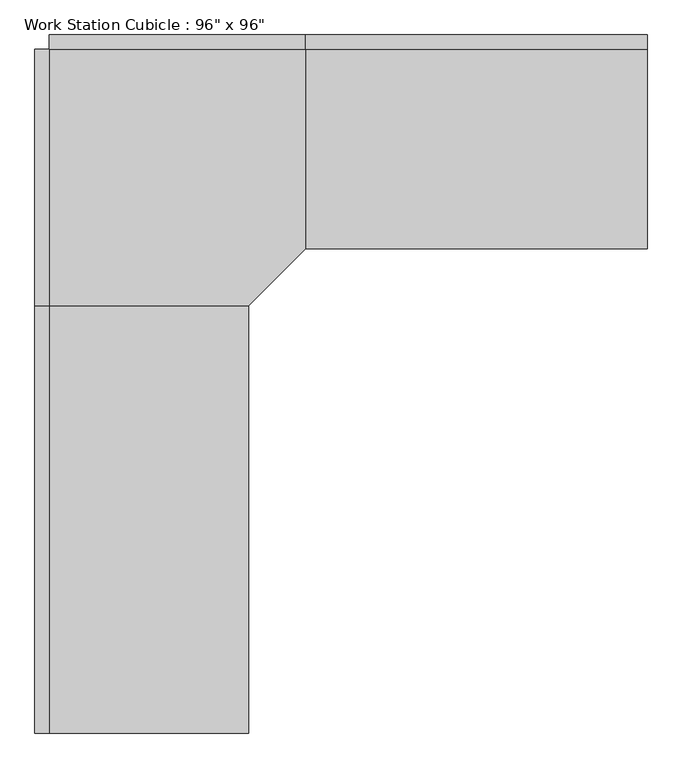
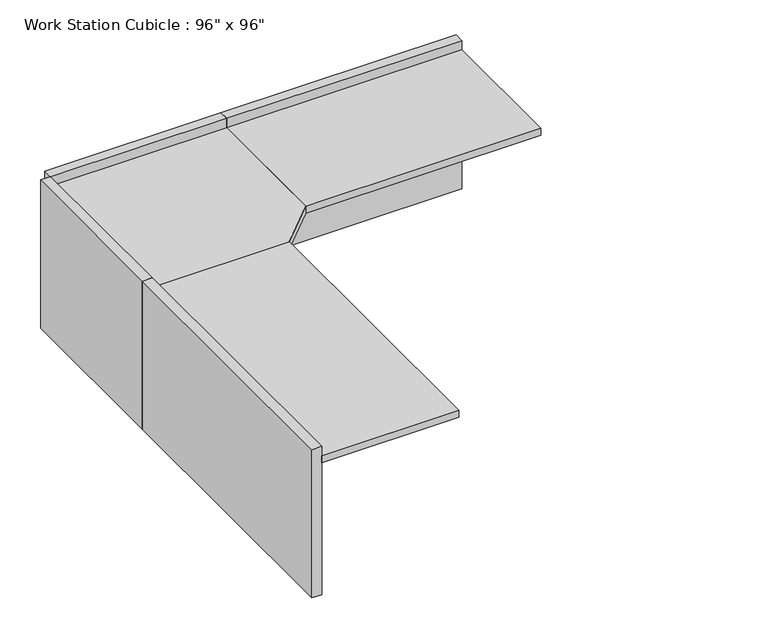
"""IFC4 building model written with IfcOpenShell, lengths in millimetres: furniture geometry."""

from ifc_helpers import new_model, si_unit, frame, origin, origin_with_axes, place, context, project, spatial, polyline, outline, extrude, source, transform, mapped, element, save


def furniture_3226db35(model_context):
    return source(origin(), model_context, "Body", "SweptSolid", [
        extrude(outline(polyline([(-80.9317522, -545.8230076), (833.4682478, -545.8230076), (833.4682478, -1257.0230076), (630.2682478, -1460.2230076), (-80.9317522, -1460.2230076), (-80.9317522, -545.8230076)])), frame((0.0, 0.0, 723.9), z_axis=(0.0, 0.0, 1.0), x_axis=(1.0, 0.0, 0.0)), (0.0, 0.0, 1.0), 38.1),
        extrude(outline(polyline([(630.2682478, -2984.2230076), (-80.9317522, -2984.2230076), (-80.9317522, -1460.2230076), (630.2682478, -1460.2230076), (630.2682478, -2984.2230076)])), frame((0.0, 0.0, 723.9), z_axis=(0.0, 0.0, 1.0), x_axis=(1.0, 0.0, 0.0)), (0.0, 0.0, 1.0), 38.1),
        extrude(outline(polyline([(2052.6682478, -1257.0230076), (833.4682478, -1257.0230076), (833.4682478, -545.8230076), (2052.6682478, -545.8230076), (2052.6682478, -1257.0230076)])), frame((0.0, 0.0, 723.9), z_axis=(0.0, 0.0, 1.0), x_axis=(1.0, 0.0, 0.0)), (0.0, 0.0, 1.0), 38.1),
        extrude(outline(polyline([(2052.6682478, -545.8230076), (833.4682478, -545.8230076), (833.4682478, -495.0230076), (2052.6682478, -495.0230076), (2052.6682478, -545.8230076)])), origin_with_axes(), (0.0, 0.0, 1.0), 812.8),
        extrude(outline(polyline([(833.4682478, -545.8230076), (-80.9317522, -545.8230076), (-80.9317522, -495.0230076), (833.4682478, -495.0230076), (833.4682478, -545.8230076)])), origin_with_axes(), (0.0, 0.0, 1.0), 812.8),
        extrude(outline(polyline([(-80.9317522, -1460.2230076), (-131.7317522, -1460.2230076), (-131.7317522, -545.8230076), (-80.9317522, -545.8230076), (-80.9317522, -1460.2230076)])), origin_with_axes(), (0.0, 0.0, 1.0), 812.8),
        extrude(outline(polyline([(-80.9317522, -2984.2230076), (-131.7317522, -2984.2230076), (-131.7317522, -1460.2230076), (-80.9317522, -1460.2230076), (-80.9317522, -2984.2230076)])), origin_with_axes(), (0.0, 0.0, 1.0), 812.8),
    ])


if __name__ == "__main__":
    model = new_model("IFC4")
    model_context = context("Model", 3, world=origin())
    ifc_project = project(units=[si_unit("LENGTHUNIT", "METRE", prefix="MILLI")], contexts=[model_context])
    site = spatial("IfcSite", under=ifc_project)
    building = spatial("IfcBuilding", under=site)
    placement = place(None, origin())
    furniture_shape = furniture_3226db35(model_context)
    element("IfcFurniture", 1, ObjectType="Work Station Cubicle : 96\" x 96\"", at=placement, inside=building, context=model_context, shape_type="MappedRepresentation", body=[
        mapped(furniture_shape, transform((0.0, 0.0, 0.0), x_axis=(1.0, 0.0, 0.0), y_axis=(0.0, 1.0, 0.0), z_axis=(0.0, 0.0, 1.0))),
    ])
    save(model, "model.ifc")

# Revit data of these elements
# Type "Work Station Cubicle : 96\" x 96\""
#   Assembly Code = "E2020"
#   Desktop Height = 2' - 6"
#   Desktop1 Width = 2' - 4"
#   Desktop2 Width = 2' - 4"
#   Panel Height = 2' - 8"
#   Panel1 Length = 5' - 0"
#   Panel2 Length = 4' - 0"
#   Cube Panel Material = Textile - Light Gray
#   Work Top Material = Laminate, Ivory, Matte
#   Default Elevation = 0
# Element 1 (IfcFurniture, "Work Station Cubicle : 96\" x 96\"")
#   Materials on its faces: "Textile - Light Gray", "Laminate, Ivory, Matte"
# Materials
#   "Textile - Light Gray": class "Fabric", colour RGB 204 204 204, transparency 0
#   "Laminate, Ivory, Matte": class "Plastic", colour RGB 247 247 239, transparency 0, Description = "Plastic Laminate - Ivory, Matte", Cost = 0
